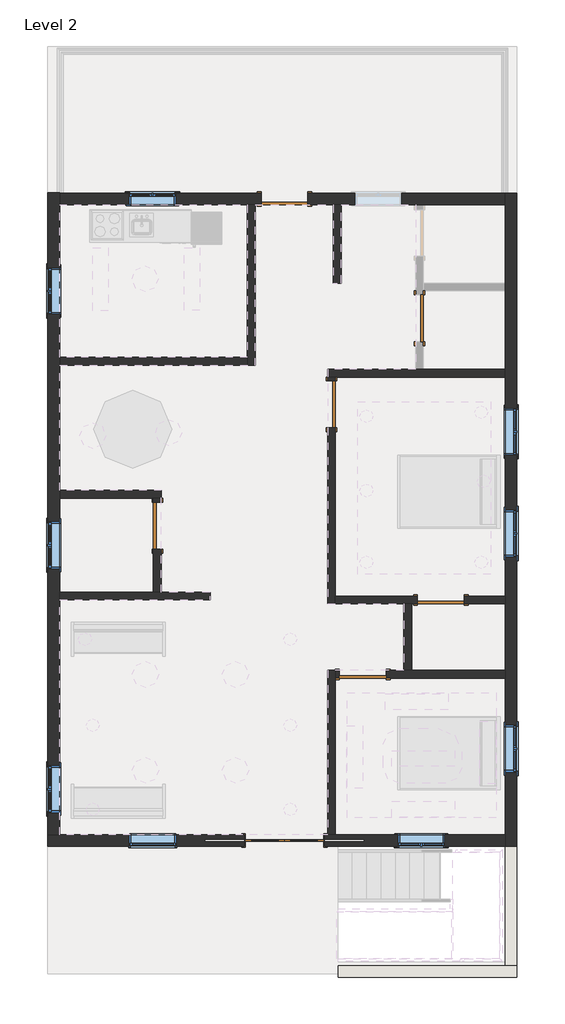
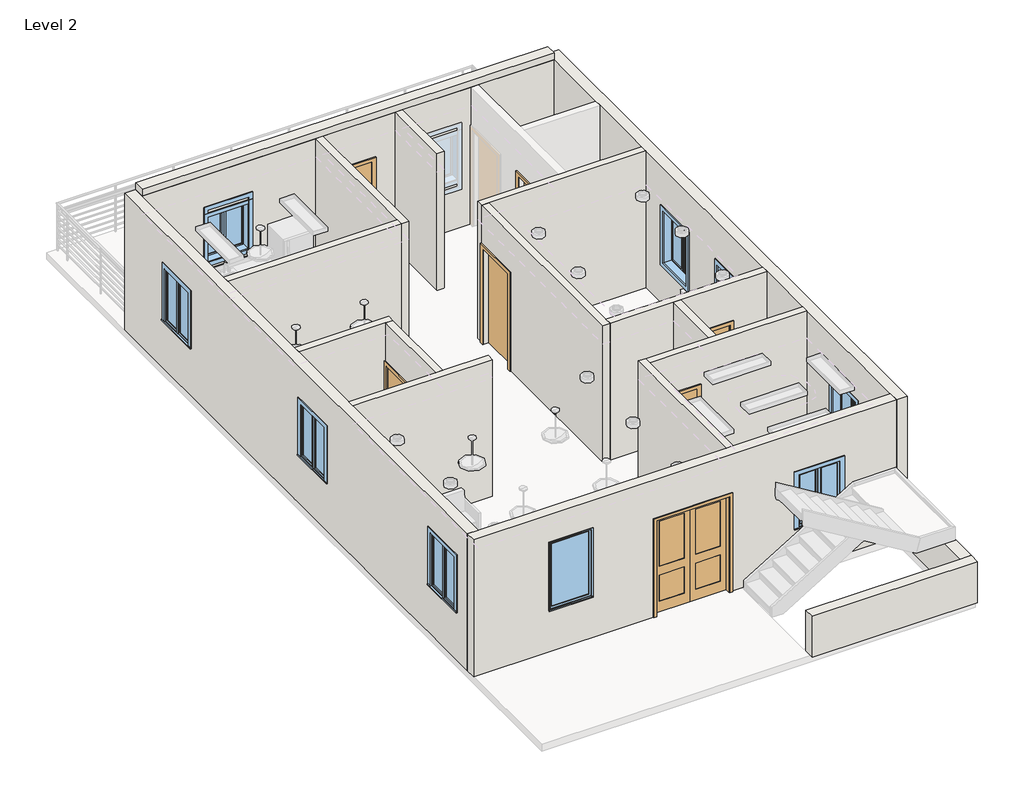
# One storey, part 1 of 3: 19 walls, 10 windows, 7 doors.
"""IFC4 building model written with IfcOpenShell, lengths in millimetres."""

from ifc_helpers import new_model, si_unit, frame, origin, place, context, project, spatial, polyline, outline, extrude, faceted_brep, transform, mapped, element, save
from components import door_53d589bd, door_0ca8825f, door_16372e1c, single_flush_single_door_686f89d2, window_419b5846, m_awning_with_trim_0915_x_1220mm_6739fb62

model = new_model("IFC4")

# Units and contexts
model_context = context("Model", 3, world=origin())
ifc_project = project(units=[si_unit("LENGTHUNIT", "METRE", prefix="MILLI")], contexts=[model_context])

# Site, building, storey
site = spatial("IfcSite", under=ifc_project)
building = spatial("IfcBuilding", under=site)
storey = spatial("IfcBuildingStorey", under=building, Name="Level 2", Elevation=3200.4)

# Doors
placement = place(None, origin())
door_shape = door_53d589bd(model_context)
element("IfcDoor", 1, ObjectType="Door-Interior-Double-Pocket-2_Panel-Wood : 60\" x 84\"", at=placement, inside=storey, context=model_context, shape_type="MappedRepresentation", body=[
    mapped(door_shape, transform((-5457.3572065, 1586.5206867, 3200.4), x_axis=(1.0, 0.0, 0.0), y_axis=(0.0, 1.0, 0.0), z_axis=(0.0, 0.0, 1.0))),
])
door_2_shape = door_0ca8825f(model_context)
element("IfcDoor", 2, ObjectType="Single-Flush : 36\" x 84\"", at=placement, inside=storey, context=model_context, shape_type="MappedRepresentation", body=[
    mapped(door_2_shape, transform((-5457.3572065, 14083.3206867, 3200.4), x_axis=(-1.0, 0.0, 0.0), y_axis=(0.0, -1.0, 0.0), z_axis=(0.0, 0.0, 1.0))),
])
door_3_shape = door_16372e1c(model_context)
element("IfcDoor", 3, ObjectType="Single-Flush : single door", at=placement, inside=storey, context=model_context, shape_type="MappedRepresentation", body=[
    mapped(door_3_shape, transform((-3933.3572065, 4825.0206867, 3200.4), x_axis=(-1.0, 0.0, 0.0), y_axis=(0.0, -1.0, 0.0), z_axis=(0.0, 0.0, 1.0))),
])
element("IfcDoor", 4, ObjectType="Single-Flush : single door", at=placement, inside=storey, context=model_context, shape_type="MappedRepresentation", body=[
    mapped(door_3_shape, transform((-2409.3572065, 6272.8206867, 3200.4), x_axis=(-1.0, 0.0, 0.0), y_axis=(0.0, -1.0, 0.0), z_axis=(0.0, 0.0, 1.0))),
])
element("IfcDoor", 5, ObjectType="Single-Flush : single door", at=placement, inside=storey, context=model_context, shape_type="MappedRepresentation", body=[
    mapped(door_3_shape, transform((-7933.8572065, 7720.6206867, 3200.4), x_axis=(0.0, 1.0, 0.0), y_axis=(-1.0, 0.0, 0.0), z_axis=(0.0, 0.0, 1.0))),
])
single_flush_single_door_shape = single_flush_single_door_686f89d2(model_context)
element("IfcDoor", 6, ObjectType="Single-Flush : single door", at=placement, inside=storey, context=model_context, shape_type="MappedRepresentation", body=[
    mapped(single_flush_single_door_shape, transform((-4542.9572065, 10082.8206867, 3200.4), x_axis=(0.0, 1.0, 0.0), y_axis=(-1.0, 0.0, 0.0), z_axis=(0.0, 0.0, 1.0))),
])
element("IfcDoor", 7, ObjectType="Single-Flush : single door", at=placement, inside=storey, context=model_context, shape_type="MappedRepresentation", body=[
    mapped(single_flush_single_door_shape, transform((-2828.4572065, 11759.2206867, 3200.4), x_axis=(0.0, 1.0, 0.0), y_axis=(-1.0, 0.0, 0.0), z_axis=(0.0, 0.0, 1.0))),
])

# Walls
element("IfcWall", 8, ObjectType="6\"", at=placement, inside=storey, context=model_context, shape_type="Brep", body=[
    faceted_brep([(-4466.7572065, 1700.8206867, 3200.4), (-4466.7572065, 4748.8206867, 3200.4), (-4466.7572065, 4901.2206867, 3200.4), (-4466.7572065, 4901.2206867, 6248.4), (-4466.7572065, 4748.8206867, 6248.4), (-4466.7572065, 1700.8206867, 6248.4), (-4619.1572065, 1700.8206867, 3200.4), (-4619.1572065, 1700.8206867, 6248.4), (-4619.1572065, 4901.2206867, 6248.4), (-4619.1572065, 4901.2206867, 3200.4)], [[[0, 1, 2, 3, 4, 5]], [[6, 7, 8, 9]], [[2, 1, 0, 6, 9]], [[5, 4, 3, 8, 7]], [[0, 5, 7, 6]], [[3, 2, 9, 8]]]),
])
element("IfcWall", 9, ObjectType="6\"", at=placement, inside=storey, context=model_context, shape_type="Brep", body=[
    faceted_brep([(-4390.5572065, 4901.2206867, 5334.0), (-4390.5572065, 4901.2206867, 3200.4), (-4466.7572065, 4901.2206867, 3200.4), (-4466.7572065, 4901.2206867, 6248.4), (-3133.2572065, 4901.2206867, 6248.4), (-2980.8572065, 4901.2206867, 6248.4), (-1158.4072065, 4901.2206867, 6248.4), (-1158.4072065, 4901.2206867, 3200.4), (-2980.8572065, 4901.2206867, 3200.4), (-3133.2572065, 4901.2206867, 3200.4), (-3476.1572065, 4901.2206867, 3200.4), (-3476.1572065, 4901.2206867, 5334.0), (-4466.7572065, 4748.8206867, 3200.4), (-4390.5572065, 4748.8206867, 3200.4), (-4390.5572065, 4748.8206867, 5334.0), (-3476.1572065, 4748.8206867, 5334.0), (-3476.1572065, 4748.8206867, 3200.4), (-1158.4072065, 4748.8206867, 3200.4), (-1158.4072065, 4748.8206867, 6248.4), (-4466.7572065, 4748.8206867, 6248.4)], [[[0, 1, 2, 3, 4, 5, 6, 7, 8, 9, 10, 11]], [[12, 13, 14, 15, 16, 17, 18, 19]], [[2, 1, 13, 12]], [[10, 9, 8, 7, 17, 16]], [[6, 5, 4, 3, 19, 18]], [[7, 6, 18, 17]], [[3, 2, 12, 19]], [[14, 13, 1, 0]], [[15, 14, 0, 11]], [[16, 15, 11, 10]]]),
])
element("IfcWall", 10, ObjectType="6\"", at=placement, inside=storey, context=model_context, shape_type="SweptSolid", body=[
    extrude(outline(polyline([(-2980.8572065, 6196.6206867), (-2980.8572065, 4901.2206867), (-3133.2572065, 4901.2206867), (-3133.2572065, 6196.6206867), (-2980.8572065, 6196.6206867)])), frame((0.0, 0.0, 3200.4), z_axis=(0.0, 0.0, 1.0), x_axis=(1.0, 0.0, 0.0)), (0.0, 0.0, 1.0), 3048.0),
])
element("IfcWall", 11, ObjectType="6\"", at=placement, inside=storey, context=model_context, shape_type="Brep", body=[
    faceted_brep([(-4466.7572065, 6349.0206867, 6248.4), (-1158.4072065, 6349.0206867, 6248.4), (-1158.4072065, 6349.0206867, 3200.4), (-1952.1572065, 6349.0206867, 3200.4), (-1952.1572065, 6349.0206867, 5334.0), (-2866.5572065, 6349.0206867, 5334.0), (-2866.5572065, 6349.0206867, 3200.4), (-4466.7572065, 6349.0206867, 3200.4), (-1158.4072065, 6196.6206867, 6248.4), (-2980.8572065, 6196.6206867, 6248.4), (-3133.2572065, 6196.6206867, 6248.4), (-4466.7572065, 6196.6206867, 6248.4), (-4466.7572065, 6196.6206867, 3200.4), (-3133.2572065, 6196.6206867, 3200.4), (-2980.8572065, 6196.6206867, 3200.4), (-2866.5572065, 6196.6206867, 3200.4), (-2866.5572065, 6196.6206867, 5334.0), (-1952.1572065, 6196.6206867, 5334.0), (-1952.1572065, 6196.6206867, 3200.4), (-1158.4072065, 6196.6206867, 3200.4)], [[[0, 1, 2, 3, 4, 5, 6, 7]], [[8, 9, 10, 11, 12, 13, 14, 15, 16, 17, 18, 19]], [[2, 19, 18, 3]], [[12, 7, 6, 15, 14, 13]], [[1, 0, 11, 10, 9, 8]], [[2, 1, 8, 19]], [[0, 7, 12, 11]], [[16, 5, 4, 17]], [[17, 4, 3, 18]], [[5, 16, 15, 6]]]),
])
element("IfcWall", 12, ObjectType="6\"", at=placement, inside=storey, context=model_context, shape_type="Brep", body=[
    faceted_brep([(-1158.4072065, 10768.6206867, 3200.4), (-2752.2572065, 10768.6206867, 3200.4), (-2904.6572065, 10768.6206867, 3200.4), (-4619.1572065, 10768.6206867, 3200.4), (-4619.1572065, 10768.6206867, 6248.4), (-2904.6572065, 10768.6206867, 6248.4), (-2752.2572065, 10768.6206867, 6248.4), (-1158.4072065, 10768.6206867, 6248.4), (-1158.4072065, 10616.2206867, 3200.4), (-1158.4072065, 10616.2206867, 6248.4), (-4466.7572065, 10616.2206867, 6248.4), (-4619.1572065, 10616.2206867, 6248.4), (-4619.1572065, 10616.2206867, 3200.4), (-4466.7572065, 10616.2206867, 3200.4)], [[[0, 1, 2, 3, 4, 5, 6, 7]], [[8, 9, 10, 11, 12, 13]], [[3, 2, 1, 0, 8, 13, 12]], [[7, 6, 5, 4, 11, 10, 9]], [[0, 7, 9, 8]], [[4, 3, 12, 11]]]),
])
element("IfcWall", 13, ObjectType="6\"", at=placement, inside=storey, context=model_context, shape_type="Brep", body=[
    faceted_brep([(-4466.7572065, 10540.0206867, 5334.0), (-4466.7572065, 10540.0206867, 3200.4), (-4466.7572065, 10616.2206867, 3200.4), (-4466.7572065, 10616.2206867, 6248.4), (-4466.7572065, 6349.0206867, 6248.4), (-4466.7572065, 6196.6206867, 6248.4), (-4466.7572065, 6196.6206867, 3200.4), (-4466.7572065, 6349.0206867, 3200.4), (-4466.7572065, 9625.6206867, 3200.4), (-4466.7572065, 9625.6206867, 5334.0), (-4619.1572065, 10616.2206867, 3200.4), (-4619.1572065, 10540.0206867, 3200.4), (-4619.1572065, 10540.0206867, 5334.0), (-4619.1572065, 9625.6206867, 5334.0), (-4619.1572065, 9625.6206867, 3200.4), (-4619.1572065, 6196.6206867, 3200.4), (-4619.1572065, 6196.6206867, 6248.4), (-4619.1572065, 10616.2206867, 6248.4)], [[[0, 1, 2, 3, 4, 5, 6, 7, 8, 9]], [[10, 11, 12, 13, 14, 15, 16, 17]], [[2, 1, 11, 10]], [[8, 7, 6, 15, 14]], [[5, 4, 3, 17, 16]], [[3, 2, 10, 17]], [[6, 5, 16, 15]], [[12, 11, 1, 0]], [[13, 12, 0, 9]], [[14, 13, 9, 8]]]),
])
element("IfcWall", 14, ObjectType="6\"", at=placement, inside=storey, context=model_context, shape_type="Brep", body=[
    faceted_brep([(-6181.2572065, 13969.0206867, 6248.4), (-6181.2572065, 13969.0206867, 3200.4), (-6181.2572065, 10997.2206867, 3200.4), (-6181.2572065, 10844.8206867, 3200.4), (-6181.2572065, 10844.8206867, 6248.4), (-6181.2572065, 10997.2206867, 6248.4), (-6028.8572065, 13969.0206867, 3200.4), (-6028.8572065, 13969.0206867, 6248.4), (-6028.8572065, 10844.8206867, 6248.4), (-6028.8572065, 10844.8206867, 3200.4)], [[[0, 1, 2, 3, 4, 5]], [[6, 7, 8, 9]], [[3, 2, 1, 6, 9]], [[0, 5, 4, 8, 7]], [[4, 3, 9, 8]], [[0, 7, 6, 1]]]),
])
element("IfcWall", 15, ObjectType="6\"", at=placement, inside=storey, context=model_context, shape_type="Brep", body=[
    faceted_brep([(-9838.8572065, 8254.0206867, 3200.4), (-8010.0572065, 8254.0206867, 3200.4), (-7857.6572065, 8254.0206867, 3200.4), (-7857.6572065, 8254.0206867, 6248.4), (-8010.0572065, 8254.0206867, 6248.4), (-9838.8572065, 8254.0206867, 6248.4), (-9838.8572065, 8406.4206867, 3200.4), (-9838.8572065, 8406.4206867, 6248.4), (-7857.6572065, 8406.4206867, 6248.4), (-7857.6572065, 8406.4206867, 3200.4)], [[[0, 1, 2, 3, 4, 5]], [[6, 7, 8, 9]], [[2, 1, 0, 6, 9]], [[5, 4, 3, 8, 7]], [[3, 2, 9, 8]], [[0, 5, 7, 6]]]),
])
element("IfcWall", 16, ObjectType="6\"", at=placement, inside=storey, context=model_context, shape_type="SweptSolid", body=[
    extrude(outline(polyline([(8254.0206867, 3200.4), (8177.8206867, 3200.4), (8177.8206867, 5334.0), (7263.4206867, 5334.0), (7263.4206867, 3200.4), (6425.2206867, 3200.4), (6425.2206867, 6248.4), (8254.0206867, 6248.4), (8254.0206867, 3200.4)])), frame((-8010.0572065, 0.0, 0.0), z_axis=(1.0, 0.0, 0.0), x_axis=(0.0, 1.0, 0.0)), (0.0, 0.0, 1.0), 152.4),
])
element("IfcWall", 17, ObjectType="6\"", at=placement, inside=storey, context=model_context, shape_type="Brep", body=[
    faceted_brep([(-6905.1572065, 6425.2206867, 3200.4), (-7857.6572065, 6425.2206867, 3200.4), (-8010.0572065, 6425.2206867, 3200.4), (-9838.8572065, 6425.2206867, 3200.4), (-9838.8572065, 6425.2206867, 6248.4), (-8010.0572065, 6425.2206867, 6248.4), (-7857.6572065, 6425.2206867, 6248.4), (-6905.1572065, 6425.2206867, 6248.4), (-6905.1572065, 6272.8206867, 3200.4), (-6905.1572065, 6272.8206867, 6248.4), (-9838.8572065, 6272.8206867, 6248.4), (-9838.8572065, 6272.8206867, 3200.4)], [[[0, 1, 2, 3, 4, 5, 6, 7]], [[8, 9, 10, 11]], [[3, 2, 1, 0, 8, 11]], [[7, 6, 5, 4, 10, 9]], [[0, 7, 9, 8]], [[4, 3, 11, 10]]]),
])
element("IfcWall", 18, ObjectType="6\"", at=placement, inside=storey, context=model_context, shape_type="SweptSolid", body=[
    extrude(outline(polyline([(-9838.8572065, 10997.2206867), (-6181.2572065, 10997.2206867), (-6181.2572065, 10844.8206867), (-9838.8572065, 10844.8206867), (-9838.8572065, 10997.2206867)])), frame((0.0, 0.0, 3200.4), z_axis=(0.0, 0.0, 1.0), x_axis=(1.0, 0.0, 0.0)), (0.0, 0.0, 1.0), 3048.0),
])
element("IfcWall", 19, ObjectType="6\"", at=placement, inside=storey, context=model_context, shape_type="SweptSolid", body=[
    extrude(outline(polyline([(-4504.8572065, 12445.0206867), (-4504.8572065, 13969.0206867), (-4352.4572065, 13969.0206867), (-4352.4572065, 12445.0206867), (-4504.8572065, 12445.0206867)])), frame((0.0, 0.0, 3200.4), z_axis=(0.0, 0.0, 1.0), x_axis=(1.0, 0.0, 0.0)), (0.0, 0.0, 1.0), 3048.0),
])
element("IfcWall", 20, ObjectType="9\"", at=placement, inside=storey, context=model_context, shape_type="Brep", body=[
    faceted_brep([(-10067.4572065, 1700.8206867, 6248.4), (-9838.8572065, 1700.8206867, 6248.4), (-4619.1572065, 1700.8206867, 6248.4), (-4466.7572065, 1700.8206867, 6248.4), (-1158.4072065, 1700.8206867, 6248.4), (-1158.4072065, 1700.8206867, 3200.4), (-4466.7572065, 1700.8206867, 3200.4), (-4619.1572065, 1700.8206867, 3200.4), (-4669.9572065, 1700.8206867, 3200.4), (-4669.9572065, 1700.8206867, 5359.4), (-6244.7572065, 1700.8206867, 5359.4), (-6244.7572065, 1700.8206867, 3200.4), (-9838.8572065, 1700.8206867, 3200.4), (-10067.4572065, 1700.8206867, 3200.4), (-3247.5572065, 1700.8206867, 5334.0), (-3247.5572065, 1700.8206867, 4114.8), (-2333.1572065, 1700.8206867, 4114.8), (-2333.1572065, 1700.8206867, 5334.0), (-8480.2572065, 1700.8206867, 5639.4), (-8480.2572065, 1700.8206867, 4115.4), (-7565.2572065, 1700.8206867, 4115.4), (-7565.2572065, 1700.8206867, 5639.4), (-1158.4072065, 1472.2206867, 6248.4), (-10067.4572065, 1472.2206867, 6248.4), (-10067.4572065, 1472.2206867, 3200.4), (-6244.7572065, 1472.2206867, 3200.4), (-6244.7572065, 1472.2206867, 5359.4), (-4669.9572065, 1472.2206867, 5359.4), (-4669.9572065, 1472.2206867, 3200.4), (-1158.4072065, 1472.2206867, 3200.4), (-3247.5572065, 1472.2206867, 5334.0), (-2333.1572065, 1472.2206867, 5334.0), (-2333.1572065, 1472.2206867, 4114.8), (-3247.5572065, 1472.2206867, 4114.8), (-8480.2572065, 1472.2206867, 5639.4), (-7565.2572065, 1472.2206867, 5639.4), (-7565.2572065, 1472.2206867, 4115.4), (-8480.2572065, 1472.2206867, 4115.4), (-4669.9572065, 1565.8831867, 3200.4), (-3907.9572065, 1565.8831867, 3200.4), (-3907.9572065, 1607.1581867, 3200.4), (-4669.9572065, 1607.1581867, 3200.4), (-6244.7572065, 1607.1581867, 3200.4), (-7006.7572065, 1607.1581867, 3200.4), (-7006.7572065, 1565.8831867, 3200.4), (-6244.7572065, 1565.8831867, 3200.4), (-3907.9572065, 1607.1581867, 5359.4), (-3907.9572065, 1565.8831867, 5359.4), (-4669.9572065, 1565.8831867, 5359.4), (-6244.7572065, 1565.8831867, 5359.4), (-7006.7572065, 1565.8831867, 5359.4), (-7006.7572065, 1607.1581867, 5359.4), (-6244.7572065, 1607.1581867, 5359.4), (-4669.9572065, 1607.1581867, 5359.4)], [[[0, 1, 2, 3, 4, 5, 6, 7, 8, 9, 10, 11, 12, 13], [14, 15, 16, 17], [18, 19, 20, 21]], [[22, 23, 24, 25, 26, 27, 28, 29], [30, 31, 32, 33], [34, 35, 36, 37]], [[5, 29, 28, 38, 39, 40, 41, 8, 7, 6]], [[24, 13, 12, 11, 42, 43, 44, 45, 25]], [[4, 3, 2, 1, 0, 23, 22]], [[15, 14, 30, 33]], [[16, 15, 33, 32]], [[17, 16, 32, 31]], [[14, 17, 31, 30]], [[46, 47, 48, 27, 26, 49, 50, 51, 52, 10, 9, 53]], [[46, 53, 41, 40]], [[53, 9, 8, 41]], [[10, 52, 42, 11]], [[52, 51, 43, 42]], [[51, 50, 44, 43]], [[50, 49, 45, 44]], [[49, 26, 25, 45]], [[27, 48, 38, 28]], [[48, 47, 39, 38]], [[47, 46, 40, 39]], [[29, 5, 4, 22]], [[19, 18, 34, 37]], [[20, 19, 37, 36]], [[21, 20, 36, 35]], [[18, 21, 35, 34]], [[0, 13, 24, 23]]]),
])
element("IfcWall", 21, ObjectType="9\"", at=placement, inside=storey, context=model_context, shape_type="Brep", body=[
    faceted_brep([(-9838.8572065, 14197.6206867, 6248.4), (-1158.4072065, 14197.6206867, 6248.4), (-1158.4072065, 14197.6206867, 3200.4), (-5000.1572065, 14197.6206867, 3200.4), (-5000.1572065, 14197.6206867, 5334.0), (-5914.5572065, 14197.6206867, 5334.0), (-5914.5572065, 14197.6206867, 3200.4), (-9838.8572065, 14197.6206867, 3200.4), (-7571.9072065, 14197.6206867, 5334.0), (-8486.3072065, 14197.6206867, 5334.0), (-8486.3072065, 14197.6206867, 4114.8), (-7571.9072065, 14197.6206867, 4114.8), (-3171.3572065, 14197.6206867, 5334.0), (-4085.7572065, 14197.6206867, 5334.0), (-4085.7572065, 14197.6206867, 4114.8), (-3171.3572065, 14197.6206867, 4114.8), (-1158.4072065, 13969.0206867, 6248.4), (-2752.2572065, 13969.0206867, 6248.4), (-2904.6572065, 13969.0206867, 6248.4), (-4352.4572065, 13969.0206867, 6248.4), (-4504.8572065, 13969.0206867, 6248.4), (-6028.8572065, 13969.0206867, 6248.4), (-6181.2572065, 13969.0206867, 6248.4), (-9838.8572065, 13969.0206867, 6248.4), (-9838.8572065, 13969.0206867, 3200.4), (-6181.2572065, 13969.0206867, 3200.4), (-6028.8572065, 13969.0206867, 3200.4), (-5914.5572065, 13969.0206867, 3200.4), (-5914.5572065, 13969.0206867, 5334.0), (-5000.1572065, 13969.0206867, 5334.0), (-5000.1572065, 13969.0206867, 3200.4), (-4504.8572065, 13969.0206867, 3200.4), (-4352.4572065, 13969.0206867, 3200.4), (-2904.6572065, 13969.0206867, 3200.4), (-2752.2572065, 13969.0206867, 3200.4), (-1158.4072065, 13969.0206867, 3200.4), (-7571.9072065, 13969.0206867, 5334.0), (-7571.9072065, 13969.0206867, 4114.8), (-8486.3072065, 13969.0206867, 4114.8), (-8486.3072065, 13969.0206867, 5334.0), (-3171.3572065, 13969.0206867, 5334.0), (-3171.3572065, 13969.0206867, 4114.8), (-4085.7572065, 13969.0206867, 4114.8), (-4085.7572065, 13969.0206867, 5334.0)], [[[0, 1, 2, 3, 4, 5, 6, 7], [8, 9, 10, 11], [12, 13, 14, 15]], [[16, 17, 18, 19, 20, 21, 22, 23, 24, 25, 26, 27, 28, 29, 30, 31, 32, 33, 34, 35], [36, 37, 38, 39], [40, 41, 42, 43]], [[24, 7, 6, 27, 26, 25]], [[2, 35, 34, 33, 32, 31, 30, 3]], [[1, 0, 23, 22, 21, 20, 19, 18, 17, 16]], [[37, 36, 8, 11]], [[38, 37, 11, 10]], [[39, 38, 10, 9]], [[36, 39, 9, 8]], [[41, 40, 12, 15]], [[42, 41, 15, 14]], [[43, 42, 14, 13]], [[40, 43, 13, 12]], [[0, 7, 24, 23]], [[35, 2, 1, 16]], [[5, 28, 27, 6]], [[28, 5, 4, 29]], [[29, 4, 3, 30]]]),
])
element("IfcWall", 22, ObjectType="9\"", at=placement, inside=storey, context=model_context, shape_type="Brep", body=[
    faceted_brep([(-1158.4072065, 14197.6206867, 6248.4), (-1158.4072065, 14197.6206867, 3352.8), (-1158.4072065, 14197.6206867, 3200.4), (-1158.4072065, 13969.0206867, 3200.4), (-1158.4072065, 12445.0206867, 3200.4), (-1158.4072065, 12292.6206867, 3200.4), (-1158.4072065, 10768.6206867, 3200.4), (-1158.4072065, 10616.2206867, 3200.4), (-1158.4072065, 6349.0206867, 3200.4), (-1158.4072065, 6196.6206867, 3200.4), (-1158.4072065, 4901.2206867, 3200.4), (-1158.4072065, 4748.8206867, 3200.4), (-1158.4072065, 1700.8206867, 3200.4), (-1158.4072065, 1472.2206867, 3200.4), (-1158.4072065, 1472.2206867, 4114.8), (-1158.4072065, 1472.2206867, 6248.4), (-1158.4072065, 1700.8206867, 6248.4), (-1158.4072065, 4748.8206867, 6248.4), (-1158.4072065, 4901.2206867, 6248.4), (-1158.4072065, 6196.6206867, 6248.4), (-1158.4072065, 6349.0206867, 6248.4), (-1158.4072065, 10616.2206867, 6248.4), (-1158.4072065, 10768.6206867, 6248.4), (-1158.4072065, 12292.6206867, 6248.4), (-1158.4072065, 12445.0206867, 6248.4), (-1158.4072065, 13969.0206867, 6248.4), (-1158.4072065, 9092.2206867, 5334.0), (-1158.4072065, 9092.2206867, 4114.8), (-1158.4072065, 10006.6206867, 4114.8), (-1158.4072065, 10006.6206867, 5334.0), (-1158.4072065, 7111.0206867, 5334.0), (-1158.4072065, 7111.0206867, 4114.8), (-1158.4072065, 8025.4206867, 4114.8), (-1158.4072065, 8025.4206867, 5334.0), (-1158.4072065, 2920.0206867, 5334.0), (-1158.4072065, 2920.0206867, 4114.8), (-1158.4072065, 3834.4206867, 4114.8), (-1158.4072065, 3834.4206867, 5334.0), (-929.8072065, 14197.6206867, 3200.4), (-929.8072065, 14197.6206867, 6248.4), (-929.8072065, 1472.2206867, 6248.4), (-929.8072065, 1472.2206867, 4114.8), (-929.8072065, 1472.2206867, 3200.4), (-929.8072065, 9092.2206867, 5334.0), (-929.8072065, 10006.6206867, 5334.0), (-929.8072065, 10006.6206867, 4114.8), (-929.8072065, 9092.2206867, 4114.8), (-929.8072065, 7111.0206867, 5334.0), (-929.8072065, 8025.4206867, 5334.0), (-929.8072065, 8025.4206867, 4114.8), (-929.8072065, 7111.0206867, 4114.8), (-929.8072065, 2920.0206867, 5334.0), (-929.8072065, 3834.4206867, 5334.0), (-929.8072065, 3834.4206867, 4114.8), (-929.8072065, 2920.0206867, 4114.8)], [[[0, 1, 2, 3, 4, 5, 6, 7, 8, 9, 10, 11, 12, 13, 14, 15, 16, 17, 18, 19, 20, 21, 22, 23, 24, 25], [26, 27, 28, 29], [30, 31, 32, 33], [34, 35, 36, 37]], [[38, 39, 40, 41, 42], [43, 44, 45, 46], [47, 48, 49, 50], [51, 52, 53, 54]], [[13, 12, 11, 10, 9, 8, 7, 6, 5, 4, 3, 2, 38, 42]], [[0, 25, 24, 23, 22, 21, 20, 19, 18, 17, 16, 15, 40, 39]], [[26, 29, 44, 43]], [[29, 28, 45, 44]], [[28, 27, 46, 45]], [[27, 26, 43, 46]], [[30, 33, 48, 47]], [[33, 32, 49, 48]], [[32, 31, 50, 49]], [[31, 30, 47, 50]], [[34, 37, 52, 51]], [[37, 36, 53, 52]], [[36, 35, 54, 53]], [[35, 34, 51, 54]], [[13, 42, 41, 40, 15, 14]], [[0, 39, 38, 2, 1]]]),
])
element("IfcWall", 23, ObjectType="9\"", at=placement, inside=storey, context=model_context, shape_type="Brep", body=[
    faceted_brep([(-9837.1451282, 14197.6206867, 6400.8), (-1158.4072065, 14197.6206867, 6400.8), (-1158.4072065, 14197.6206867, 6248.4), (-1158.4072065, 14197.6206867, 3352.8), (-5000.1572065, 14197.6206867, 3352.8), (-5000.1572065, 14197.6206867, 5334.0), (-5914.5572065, 14197.6206867, 5334.0), (-5914.5572065, 14197.6206867, 3352.8), (-9838.8572065, 14197.6206867, 3352.8), (-9838.8572065, 14197.6206867, 6248.4), (-9837.1451282, 14197.6206867, 6248.4), (-7571.9072065, 14197.6206867, 5486.4), (-8486.3072065, 14197.6206867, 5486.4), (-8486.3072065, 14197.6206867, 4267.2), (-7571.9072065, 14197.6206867, 4267.2), (-3171.3572065, 14197.6206867, 5486.4), (-4085.7572065, 14197.6206867, 5486.4), (-4085.7572065, 14197.6206867, 4267.2), (-3171.3572065, 14197.6206867, 4267.2), (-1158.4072065, 13969.0206867, 6400.8), (-9837.1451282, 13969.0206867, 6400.8), (-9837.1451282, 13969.0206867, 6248.4), (-9838.8572065, 13969.0206867, 6248.4), (-9838.8572065, 13969.0206867, 3352.8), (-5914.5572065, 13969.0206867, 3352.8), (-5914.5572065, 13969.0206867, 5334.0), (-5000.1572065, 13969.0206867, 5334.0), (-5000.1572065, 13969.0206867, 3352.8), (-1158.4072065, 13969.0206867, 3352.8), (-7571.9072065, 13969.0206867, 5486.4), (-7571.9072065, 13969.0206867, 4267.2), (-8486.3072065, 13969.0206867, 4267.2), (-8486.3072065, 13969.0206867, 5486.4), (-3171.3572065, 13969.0206867, 5486.4), (-3171.3572065, 13969.0206867, 4267.2), (-4085.7572065, 13969.0206867, 4267.2), (-4085.7572065, 13969.0206867, 5486.4)], [[[0, 1, 2, 3, 4, 5, 6, 7, 8, 9, 10], [11, 12, 13, 14], [15, 16, 17, 18]], [[19, 20, 21, 22, 23, 24, 25, 26, 27, 28], [29, 30, 31, 32], [33, 34, 35, 36]], [[23, 8, 7, 24]], [[3, 28, 27, 4]], [[1, 0, 20, 19]], [[30, 29, 11, 14]], [[31, 30, 14, 13]], [[32, 31, 13, 12]], [[29, 32, 12, 11]], [[34, 33, 15, 18]], [[35, 34, 18, 17]], [[36, 35, 17, 16]], [[33, 36, 16, 15]], [[10, 9, 22, 21]], [[8, 23, 22, 9]], [[20, 0, 10, 21]], [[28, 3, 2, 1, 19]], [[6, 25, 24, 7]], [[25, 6, 5, 26]], [[26, 5, 4, 27]]]),
])
element("IfcWall", 24, ObjectType="9\"", at=placement, inside=storey, context=model_context, shape_type="Brep", body=[
    faceted_brep([(-9838.8572065, 1700.8206867, 3200.4), (-9838.8572065, 6272.8206867, 3200.4), (-9838.8572065, 6425.2206867, 3200.4), (-9838.8572065, 8254.0206867, 3200.4), (-9838.8572065, 8406.4206867, 3200.4), (-9838.8572065, 10844.8206867, 3200.4), (-9838.8572065, 10997.2206867, 3200.4), (-9838.8572065, 13969.0206867, 3200.4), (-9838.8572065, 14197.6206867, 3200.4), (-9838.8572065, 14210.3206867, 3200.4), (-9838.8572065, 14210.3206867, 6248.4), (-9838.8572065, 14197.6206867, 6248.4), (-9838.8572065, 13969.0206867, 6248.4), (-9838.8572065, 10997.2206867, 6248.4), (-9838.8572065, 10844.8206867, 6248.4), (-9838.8572065, 8406.4206867, 6248.4), (-9838.8572065, 8254.0206867, 6248.4), (-9838.8572065, 6425.2206867, 6248.4), (-9838.8572065, 6272.8206867, 6248.4), (-9838.8572065, 1700.8206867, 6248.4), (-9838.8572065, 3047.0206867, 5486.4), (-9838.8572065, 3047.0206867, 4267.2), (-9838.8572065, 2132.6206867, 4267.2), (-9838.8572065, 2132.6206867, 5486.4), (-9838.8572065, 7796.8206867, 5486.4), (-9838.8572065, 7796.8206867, 4267.2), (-9838.8572065, 6882.4206867, 4267.2), (-9838.8572065, 6882.4206867, 5486.4), (-9838.8572065, 12749.8206867, 5486.4), (-9838.8572065, 12749.8206867, 4267.2), (-9838.8572065, 11835.4206867, 4267.2), (-9838.8572065, 11835.4206867, 5486.4), (-10067.4572065, 1700.8206867, 3200.4), (-10067.4572065, 1700.8206867, 6248.4), (-10067.4572065, 14210.3206867, 6248.4), (-10067.4572065, 14210.3206867, 3200.4), (-10067.4572065, 3047.0206867, 5486.4), (-10067.4572065, 2132.6206867, 5486.4), (-10067.4572065, 2132.6206867, 4267.2), (-10067.4572065, 3047.0206867, 4267.2), (-10067.4572065, 7796.8206867, 5486.4), (-10067.4572065, 6882.4206867, 5486.4), (-10067.4572065, 6882.4206867, 4267.2), (-10067.4572065, 7796.8206867, 4267.2), (-10067.4572065, 12749.8206867, 5486.4), (-10067.4572065, 11835.4206867, 5486.4), (-10067.4572065, 11835.4206867, 4267.2), (-10067.4572065, 12749.8206867, 4267.2)], [[[0, 1, 2, 3, 4, 5, 6, 7, 8, 9, 10, 11, 12, 13, 14, 15, 16, 17, 18, 19], [20, 21, 22, 23], [24, 25, 26, 27], [28, 29, 30, 31]], [[32, 33, 34, 35], [36, 37, 38, 39], [40, 41, 42, 43], [44, 45, 46, 47]], [[9, 8, 7, 6, 5, 4, 3, 2, 1, 0, 32, 35]], [[10, 9, 35, 34]], [[19, 18, 17, 16, 15, 14, 13, 12, 11, 10, 34, 33]], [[20, 23, 37, 36]], [[23, 22, 38, 37]], [[22, 21, 39, 38]], [[21, 20, 36, 39]], [[24, 27, 41, 40]], [[27, 26, 42, 41]], [[26, 25, 43, 42]], [[25, 24, 40, 43]], [[28, 31, 45, 44]], [[31, 30, 46, 45]], [[30, 29, 47, 46]], [[29, 28, 44, 47]], [[0, 19, 33, 32]]]),
])
element("IfcWall", 25, ObjectType="9\"", at=placement, inside=storey, context=model_context, shape_type="SweptSolid", body=[
    extrude(outline(polyline([(-1158.4072065, -851.8793133), (-1158.4072065, 1472.2206867), (-929.8072065, 1472.2206867), (-929.8072065, -851.8793133), (-1158.4072065, -851.8793133)])), frame((0.0, 0.0, 3200.4), z_axis=(0.0, 0.0, 1.0), x_axis=(1.0, 0.0, 0.0)), (0.0, 0.0, 1.0), 914.4),
])
element("IfcWall", 26, ObjectType="9\"", at=placement, inside=storey, context=model_context, shape_type="Brep", body=[
    faceted_brep([(-4409.6072065, -1080.4793133, 3200.4), (-929.8072065, -1080.4793133, 3200.4), (-929.8072065, -1080.4793133, 4114.8), (-4409.6072065, -1080.4793133, 4114.8), (-4409.6072065, -851.8793133, 3200.4), (-4409.6072065, -851.8793133, 4114.8), (-1158.4072065, -851.8793133, 4114.8), (-929.8072065, -851.8793133, 4114.8), (-929.8072065, -851.8793133, 3200.4), (-1158.4072065, -851.8793133, 3200.4)], [[[0, 1, 2, 3]], [[4, 5, 6, 7, 8, 9]], [[1, 0, 4, 9, 8]], [[3, 2, 7, 6, 5]], [[0, 3, 5, 4]], [[2, 1, 8, 7]]]),
])

# Windows
window_shape = window_419b5846(model_context)
element("IfcWindow", 27, ObjectType="Casement Dbl with Trim : 48\" x 48\"", at=placement, inside=storey, context=model_context, shape_type="MappedRepresentation", body=[
    mapped(window_shape, transform((-8029.1072065, 14064.2706867, 3200.4), x_axis=(1.0, 0.0, 0.0), y_axis=(0.0, 1.0, 0.0), z_axis=(0.0, 0.0, 1.0))),
])
element("IfcWindow", 28, ObjectType="Casement Dbl with Trim : 48\" x 48\"", at=placement, inside=storey, context=model_context, shape_type="MappedRepresentation", body=[
    mapped(window_shape, transform((-1063.1572065, 9549.4206867, 3200.4), x_axis=(0.0, -1.0, 0.0), y_axis=(1.0, 0.0, 0.0), z_axis=(0.0, 0.0, 1.0))),
])
element("IfcWindow", 29, ObjectType="Casement Dbl with Trim : 48\" x 48\"", at=placement, inside=storey, context=model_context, shape_type="MappedRepresentation", body=[
    mapped(window_shape, transform((-1063.1572065, 7568.2206867, 3200.4), x_axis=(0.0, -1.0, 0.0), y_axis=(1.0, 0.0, 0.0), z_axis=(0.0, 0.0, 1.0))),
])
element("IfcWindow", 30, ObjectType="Casement Dbl with Trim : 48\" x 48\"", at=placement, inside=storey, context=model_context, shape_type="MappedRepresentation", body=[
    mapped(window_shape, transform((-1063.1572065, 3377.2206867, 3200.4), x_axis=(0.0, -1.0, 0.0), y_axis=(1.0, 0.0, 0.0), z_axis=(0.0, 0.0, 1.0))),
])
element("IfcWindow", 31, ObjectType="Casement Dbl with Trim : 48\" x 48\"", at=placement, inside=storey, context=model_context, shape_type="MappedRepresentation", body=[
    mapped(window_shape, transform((-2790.3572065, 1605.5706867, 3200.4), x_axis=(-1.0, 0.0, 0.0), y_axis=(0.0, -1.0, 0.0), z_axis=(0.0, 0.0, 1.0))),
])
element("IfcWindow", 32, ObjectType="Casement Dbl with Trim : 48\" x 48\"", at=placement, inside=storey, context=model_context, shape_type="MappedRepresentation", body=[
    mapped(window_shape, transform((-9934.1072065, 2589.8206867, 3352.8), x_axis=(0.0, 1.0, 0.0), y_axis=(-1.0, 0.0, 0.0), z_axis=(0.0, 0.0, 1.0))),
])
element("IfcWindow", 33, ObjectType="Casement Dbl with Trim : 48\" x 48\"", at=placement, inside=storey, context=model_context, shape_type="MappedRepresentation", body=[
    mapped(window_shape, transform((-9934.1072065, 7339.6206867, 3352.8), x_axis=(0.0, 1.0, 0.0), y_axis=(-1.0, 0.0, 0.0), z_axis=(0.0, 0.0, 1.0))),
])
element("IfcWindow", 34, ObjectType="Casement Dbl with Trim : 48\" x 48\"", at=placement, inside=storey, context=model_context, shape_type="MappedRepresentation", body=[
    mapped(window_shape, transform((-9934.1072065, 12292.6206867, 3352.8), x_axis=(0.0, 1.0, 0.0), y_axis=(-1.0, 0.0, 0.0), z_axis=(0.0, 0.0, 1.0))),
])
element("IfcWindow", 35, ObjectType="Casement Dbl with Trim : 48\" x 48\"", at=placement, inside=storey, context=model_context, shape_type="MappedRepresentation", body=[
    mapped(window_shape, transform((-8029.1072065, 14064.2706867, 3352.8), x_axis=(1.0, 0.0, 0.0), y_axis=(0.0, 1.0, 0.0), z_axis=(0.0, 0.0, 1.0))),
])
m_awning_with_trim_0915_x_1220mm_shape = m_awning_with_trim_0915_x_1220mm_6739fb62(model_context)
element("IfcWindow", 36, ObjectType="M_Awning with Trim : 0915 x 1220mm", at=placement, inside=storey, context=model_context, shape_type="MappedRepresentation", body=[
    mapped(m_awning_with_trim_0915_x_1220mm_shape, transform((-8022.7572065, 1586.5206867, 3200.4), x_axis=(-1.0, 0.0, 0.0), y_axis=(0.0, -1.0, 0.0), z_axis=(0.0, 0.0, 1.0))),
])

save(model, "model.ifc")

# Revit data of these elements
# Type "Door-Interior-Double-Pocket-2_Panel-Wood : 60\" x 84\""
#   Type Mark = "12"
#   Assembly Code = "C1020300"
#   Analytic Construction = "Wooden"
#   Top Rail = 0' - 4 11/16"
#   Thickness = 0' - 1 3/8"
#   Thermal Resistance (R) = 2.5876 (h·ft²·°F)/BTU
#   Stiles = 0' - 4 3/4"
#   Rough Width = 10' - 2"
#   Rough Height = 7' - 4 1/2"
#   Panel Width = 2' - 6"
#   Lock Rail = 0' - 7 1/2"
#   Location [instance default] = 2' - 7"
#   Height = 7' - 0"
#   Width = 5' - 0"
#   Heat Transfer Coefficient (U) = 0.3865 BTU/(h·ft²·°F)
#   Bottom Rail = 0' - 9 1/8"
#   Panel Open [instance default] = no
#   Trim Material = Cherry
#   Panel Material = Cherry
#   Frame Material = Cherry
#   Visual Light Transmittance = 0
#   Solar Heat Gain Coefficient = 0
#   Wall Closure = (empty or 0)
#   Function = (empty or 0)
# Type "Single-Flush : 36\" x 84\""
#   Type Mark = "1"
#   Construction Type Id = "MDOOR"
#   Assembly Code = "C1020"
#   Analytic Construction = "Metal"
#   Thickness = 0' - 2"
#   Heat Transfer Coefficient (U) = 0.651978 BTU/(h·ft²·°F)
#   Height = 7' - 0"
#   Trim Projection Ext = 0' - 1"
#   Trim Projection Int = 0' - 1"
#   Trim Width = 0' - 3"
#   Width = 3' - 0"
#   Define Thermal Properties by = 1
#   Door Material = Door - Panel
#   Frame Material = Door - Frame
#   Visual Light Transmittance = 0
#   Solar Heat Gain Coefficient = 0
#   Function = (empty or 0)
#   Wall Closure = (empty or 0)
# Type "Single-Flush : single door"
#   Type Mark = "11"
#   Construction Type Id = "MDOOR"
#   Assembly Code = "C1020"
#   Analytic Construction = "Metal"
#   Thickness = 0' - 2"
#   Heat Transfer Coefficient (U) = 0.651978 BTU/(h·ft²·°F)
#   Height = 7' - 0"
#   Trim Projection Ext = 0' - 1"
#   Trim Projection Int = 0' - 1"
#   Trim Width = 0' - 3"
#   Width = 3' - 0"
#   Define Thermal Properties by = 1
#   Door Material = Door - Panel
#   Frame Material = Door - Frame
#   Visual Light Transmittance = 0
#   Solar Heat Gain Coefficient = 0
#   Function = (empty or 0)
#   Wall Closure = (empty or 0)
# Type "6\""
#   Assembly Code = "B2010"
#   Layers, outside or top first: 0' - 6" "interior walls" (function 1)
# Type "9\""
#   Assembly Code = "B2010"
#   Layers, outside or top first: 0' - 9" "ext walls" (function 1)
# Type "Casement Dbl with Trim : 48\" x 48\""
#   Type Mark = "10"
#   Construction Type Id = "GSP4R"
#   Assembly Code = "B2020100"
#   Analytic Construction = "1/8 in Pilkington single glazing"
#   Visual Light Transmittance = 0.9
#   Solar Heat Gain Coefficient = 0.78
#   Heat Transfer Coefficient (U) = 0.6496 BTU/(h·ft²·°F)
#   Height = 4' - 0"
#   Default Sill Height = 3' - 0"
#   Trim Projection - Ext. = 0' - 0 1/2"
#   Trim Projection - Int. = 0' - 0 3/4"
#   Trim Width - Exterior = 0' - 3 1/2"
#   Trim Width - Interior = 0' - 3 1/2"
#   Width = 3' - 0"
#   Window Inset = 0' - 0 3/4"
#   Define Thermal Properties by = 1
#   Glass Pane Material = Glass
#   Sash Material = Sash
#   Trim Exterior Material = Trim
#   Trim Interior Material = Trim
#   Wall Closure = (empty or 0)
# Type "M_Awning with Trim : 0915 x 1220mm"
#   Type Mark = "13"
#   Construction Type Id = "GSP4R"
#   Analytic Construction = "1/8 in Pilkington single glazing"
#   Visual Light Transmittance = 0.9
#   Solar Heat Gain Coefficient = 0.78
#   Heat Transfer Coefficient (U) = 0.6496 BTU/(h·ft²·°F)
#   Height = 5' - 0"
#   Default Sill Height = 3' - 0.02362"
#   Trim Projection - Ext. = 0' - 0.51181"
#   Trim Projection - Int. = 0' - 0.74803"
#   Trim Width - Exterior = 0' - 1"
#   Trim Width - Interior = 0' - 1"
#   Width = 3' - 0.02362"
#   Window Inset = 0' - 0.74803"
#   Define Thermal Properties by = 1
#   Glass Pane Material = Glass
#   Sash = Sash
#   Trim Exterior Material = Trim
#   Trim Interior Material = Trim
#   Wall Closure = (empty or 0)
# Element 1 (IfcDoor, "Door-Interior-Double-Pocket-2_Panel-Wood : 60\" x 84\"")
#   Location = 2' - 7"
#   Panel Open = no
#   Phase Created = New Construction
#   Materials on its faces: "Cherry"
# Element 2 (IfcDoor, "Single-Flush : 36\" x 84\"")
#   Phase Created = New Construction
#   Materials on its faces: "Door - Frame", "Door - Panel"
# Elements 3, 4, 5, 6, 7 (IfcDoor, "Single-Flush : single door")
#   Phase Created = New Construction
#   Materials on its faces: "Door - Frame", "Door - Panel"
# Elements 8, 9, 10, 11, 12, 13, 14, 15, 16, 17, 18, 19 (IfcWall, "6\"")
#   Top Offset = 0' - 0"
#   Base Offset = 0' - 0"
#   Unconnected Height = 10' - 0"
#   wall height = 10' - 0"
#   Phase Created = New Construction
#   Base Constraint = Level 2
#   Materials on its faces: "interior walls"
# Elements 20, 21, 22 (IfcWall, "9\"")
#   Top Offset = 0' - 0"
#   Base Offset = 0' - 0"
#   Unconnected Height = 10' - 0"
#   wall height = 10' - 0"
#   Phase Created = New Construction
#   Base Constraint = Level 2
#   Materials on its faces: "ext walls"
# Element 23 (IfcWall, "9\"")
#   built-in parameter 1001111 = 0' - 6"
#   Top Offset = 0' - 0"
#   Base Offset = 0' - 6"
#   Unconnected Height = 10' - 0"
#   wall height = 10' - 0"
#   Phase Created = New Construction
#   Base Constraint = Level 2
#   Materials on its faces: "ext walls"
# Element 24 (IfcWall, "9\"")
#   built-in parameter 1001111 = 0' - 0"
#   Top Offset = 0' - 0"
#   Base Offset = 0' - 0"
#   Unconnected Height = 10' - 0"
#   wall height = 10' - 0"
#   Phase Created = New Construction
#   Base Constraint = Level 2
#   Materials on its faces: "ext walls"
# Element 25 (IfcWall, "9\"")
#   built-in parameter 1001111 = 0' - 0"
#   Top Offset = 0' - 0"
#   Base Offset = 0' - 0"
#   Unconnected Height = 3' - 0"
#   wall height = 3' - 0"
#   Phase Created = New Construction
#   Base Constraint = Level 2
#   Materials on its faces: "ext walls"
# Element 26 (IfcWall, "9\"")
#   Top Offset = 0' - 0"
#   Base Offset = 0' - 0"
#   Unconnected Height = 3' - 0"
#   wall height = 3' - 0"
#   Phase Created = New Construction
#   Base Constraint = Level 2
#   Materials on its faces: "ext walls"
# Element 27 (IfcWindow, "Casement Dbl with Trim : 48\" x 48\"")
#   Mark = "19"
#   Phase Created = New Construction
#   Materials on its faces: "Sash", "Trim", "Glass"
# Element 28 (IfcWindow, "Casement Dbl with Trim : 48\" x 48\"")
#   Mark = "21"
#   Phase Created = New Construction
#   Materials on its faces: "Sash", "Trim", "Glass"
# Element 29 (IfcWindow, "Casement Dbl with Trim : 48\" x 48\"")
#   Mark = "22"
#   Phase Created = New Construction
#   Materials on its faces: "Sash", "Trim", "Glass"
# Element 30 (IfcWindow, "Casement Dbl with Trim : 48\" x 48\"")
#   Mark = "23"
#   Phase Created = New Construction
#   Materials on its faces: "Sash", "Trim", "Glass"
# Element 31 (IfcWindow, "Casement Dbl with Trim : 48\" x 48\"")
#   Mark = "24"
#   Phase Created = New Construction
#   Materials on its faces: "Sash", "Trim", "Glass"
# Element 32 (IfcWindow, "Casement Dbl with Trim : 48\" x 48\"")
#   Mark = "25"
#   Phase Created = New Construction
#   Materials on its faces: "Sash", "Trim", "Glass"
# Element 33 (IfcWindow, "Casement Dbl with Trim : 48\" x 48\"")
#   Mark = "26"
#   Phase Created = New Construction
#   Materials on its faces: "Sash", "Trim", "Glass"
# Element 34 (IfcWindow, "Casement Dbl with Trim : 48\" x 48\"")
#   Mark = "27"
#   Phase Created = New Construction
#   Materials on its faces: "Sash", "Trim", "Glass"
# Element 35 (IfcWindow, "Casement Dbl with Trim : 48\" x 48\"")
#   Mark = "28"
#   Phase Created = New Construction
#   Materials on its faces: "Sash", "Trim", "Glass"
# Element 36 (IfcWindow, "M_Awning with Trim : 0915 x 1220mm")
#   Mark = "45"
#   Phase Created = New Construction
#   Materials on its faces: "Trim", "Sash", "Glass"
# Materials
#   "Cherry": class "Wood", colour RGB 226 177 128, transparency 0, Description = "Prunus Serotina", Cost = 0
#   "Door - Panel": class "Wood", colour RGB 210 159 95, transparency 0
#   "Door - Frame": colour RGB 118 70 51, transparency 0
#   "interior walls": class "Generic", colour RGB 114 147 63, transparency 0, Cost = 0
#   "ext walls": class "Generic", colour RGB 120 120 120, transparency 0, Cost = 0
#   "Glass": class "Glass", colour RGB 0 128 192, transparency 0.75, Description = "Soda Lime Glass", Cost = 0
#   "Sash": class "Wood", colour RGB 224 178 126, transparency 0
#   "Trim": class "Wood", colour RGB 224 178 126, transparency 0
